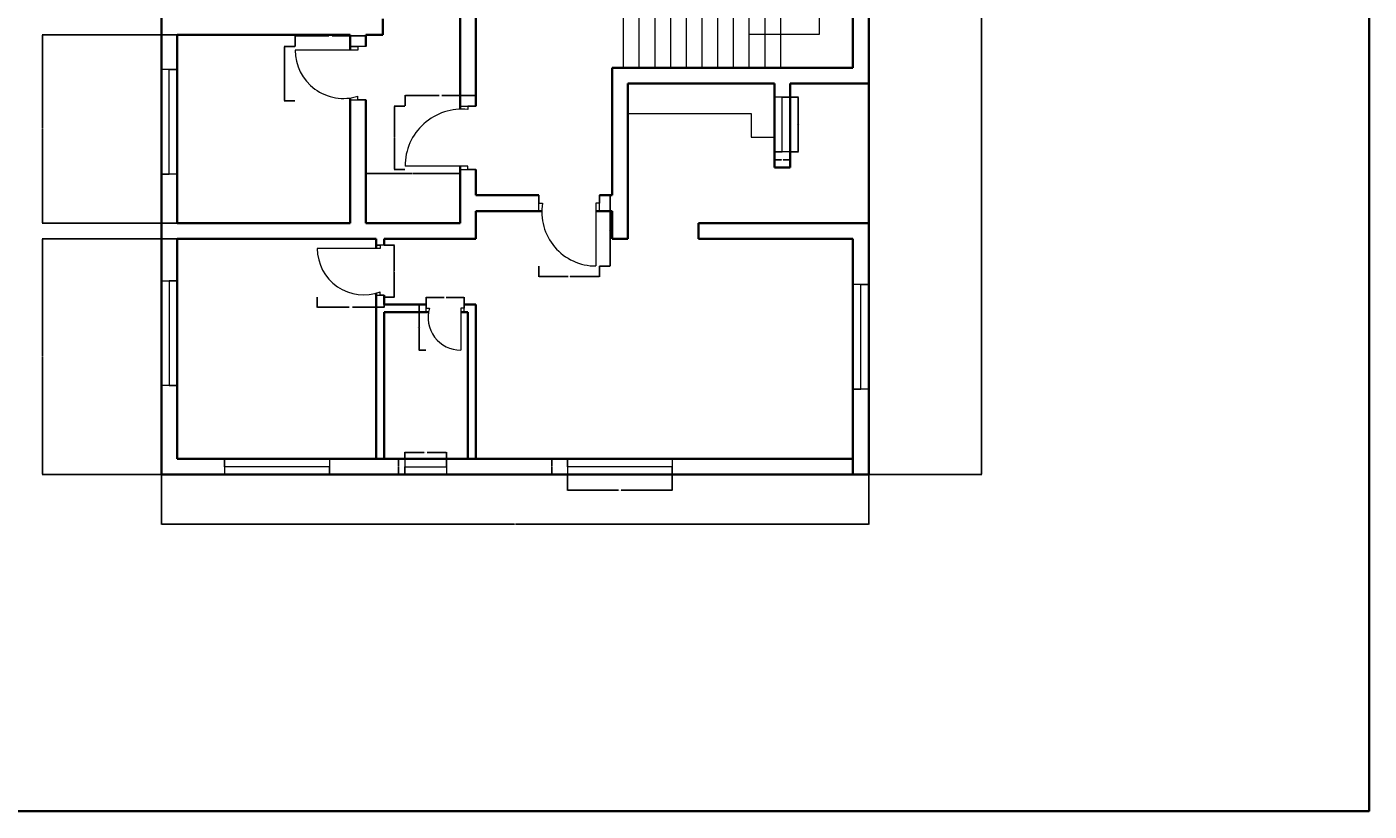
# Model space of a CAD drawing. Units: inches. Extents: x 1955 to 3324, y 980 to 3129.
# Tile 7 of 11: x 2555 to 3324, y 1704 to 2153. Entities that reach past the tile are written whole.
import ezdxf

# ---------------------------------------------------------------- set-up
doc = ezdxf.new("R2010")
doc.units = ezdxf.units.IN
for name, color, linetype, lineweight in [('A-ANNO-DIMS', 2, 'Continuous', 18), ('A-ANNO-TTLB', 7, 'Continuous', 35), ('A-DOOR', 3, 'Continuous', 18), ('A-FLOR-CASE', 8, 'Continuous', 18), ('A-FLOR-STRS', 7, 'Continuous', 18), ('A-GLAZ', 4, 'Continuous', 18), ('A-WALL', 7, 'Continuous', 35)]:
    doc.layers.add(name, color=color, linetype=linetype, lineweight=lineweight)
doc.styles.get("Standard").update_dxf_attribs({"font": 'arial.ttf'})
doc.dimstyles.get("Standard").update_dxf_attribs({"dimtxt": 0.18, "dimasz": 0.18, "dimexe": 0.18, "dimexo": 0.0625, "dimgap": 0.09, "dimtad": 0, "dimtih": 1, "dimtoh": 1, "dimdec": 4, "dimzin": 0, "dimdsep": 46, "dimtxsty": 'Standard', "dimcen": 0.09, "dimadec": 0, "dimazin": 0, "dimtfac": 1, "dimtdec": 4, "dimtofl": 0, "dimtmove": 0, "dimatfit": 3, "dimfxl": 1, "dimtolj": 1, "dimtzin": 0, "dimarcsym": 0})

# ---------------------------------------------------------------- blocks, each defined once
blk = doc.blocks.new('DOOR-UNIT-W')
for p, q in [((31.5, 36.35), (40.5, 36.35)), ((40.5, 36.35), (36, 36.35)), ((36, 36.35), (36, 34.35)), ((36, 2), (0, 2)), ((31.5, 0), (40.5, 0)), ((36, 0), (36, 2)), ((40.5, 0), (36, 0))]:
    blk.add_line(p, q)
blk.add_arc((32.53, 2), 32.53, 83.87992, 180)
blk = doc.blocks.new('DOOR-BED-S')
for p, q in [((36, 26.66), (0, 26.66)), ((38.25, 28.66), (33.75, 28.66)), ((33.75, 28.66), (36, 28.66)), ((36, 28.66), (36, 26.66)), ((36, 0), (36, 2)), ((33.75, 0), (38.25, 0)), ((38.25, 0), (36, 0))]:
    blk.add_line(p, q)
blk.add_arc((26.45, 26.66), 26.45, 180, 291.17181)
blk = doc.blocks.new('DOOR-WC-S')
for p, q in [((0, 21.75), (0, 26.25)), ((0, 26.25), (0, 24)), ((0, 24), (2, 24)), ((21.9, 24), (19.9, 24)), ((19.9, 24), (19.9, 0)), ((21.9, 21.75), (21.9, 26.25)), ((21.9, 26.25), (21.9, 24))]:
    blk.add_line(p, q)
blk.add_arc((19.9, 18.68), 18.68, 163.43907, 270)
blk = doc.blocks.new('DOOR-UNIT-S')
for p, q in [((0, 31.5), (0, 40.5)), ((0, 40.5), (0, 36)), ((34.6, 31.5), (34.6, 40.5)), ((34.6, 40.5), (34.6, 36)), ((0, 36), (2, 36)), ((34.6, 36), (32.6, 36)), ((32.6, 36), (32.6, 0))]:
    blk.add_line(p, q)
blk.add_arc((32.6, 31.01), 31.01, 170.73008, 270)
blk = doc.blocks.new('DOOR-BED-W')
for p, q in [((36, 28.47), (0, 28.47)), ((40.5, 30.47), (31.5, 30.47)), ((31.5, 30.47), (36, 30.47)), ((36, 30.47), (36, 28.47)), ((31.5, 0), (40.5, 0)), ((36, 0), (36, 2)), ((40.5, 0), (36, 0))]:
    blk.add_line(p, q)
blk.add_arc((27.73, 28.47), 27.73, 180, 287.3494)
blk = doc.blocks.new('WIN-PLAN-60-A')
for p, q in [((0, 60), (9, 60)), ((9, 60), (4.5, 60)), ((4.5, 60), (4.5, 0)), ((4.5, 0), (0, 0)), ((0, 0), (9, 0))]:
    blk.add_line(p, q)
blk = doc.blocks.new('WIN-PLAN-60-B')
for p, q in [((0, 0), (0, 9)), ((0, 9), (0, 4.5)), ((60, 4.5), (60, 9)), ((60, 9), (60, 0)), ((0, 4.5), (60, 4.5))]:
    blk.add_line(p, q)
blk = doc.blocks.new('WIN-PLAN-24-A')
for p, q in [((0, 9), (0, 0)), ((24, 4.5), (24, 9)), ((24, 9), (24, 0)), ((0, 0), (0, 4.5)), ((0, 4.5), (24, 4.5))]:
    blk.add_line(p, q)
blk = doc.blocks.new('WIN-PLAN-31')
for p, q in [((0, 31.31), (9, 31.31)), ((9, 31.31), (4.5, 31.31)), ((4.5, 31.31), (4.5, 0)), ((4.5, 0), (0, 0)), ((0, 0), (9, 0))]:
    blk.add_line(p, q)
blk = doc.blocks.new('COUNTER-L-S')
for p, q in [((0, 13.55), (70.65, 13.55)), ((70.65, 13.55), (70.65, 0)), ((70.65, 0), (83.99, 0))]:
    blk.add_line(p, q)
blk = doc.blocks.new('STAIR-RETURN-FLIGHT')
for p, q in [((17.37, 47), (17.37, 94)), ((17.37, 94), (17.37, 0)), ((26.37, 94), (26.37, 0)), ((35.37, 94), (35.37, 0)), ((44.37, 94), (44.37, 0)), ((53.37, 94), (53.37, 0)), ((62.37, 94), (62.37, 0)), ((71.37, 94), (71.37, 0)), ((80.37, 94), (80.37, 0)), ((89.37, 94), (89.37, 0)), ((98.37, 94), (98.37, 0)), ((107.37, 94), (107.37, 0)), ((0, 68.91), (129.63, 68.91)), ((129.63, 68.91), (129.63, 19.03)), ((107.37, 47), (17.37, 47)), ((129.63, 19.03), (89.37, 19.03))]:
    blk.add_line(p, q)
blk = doc.blocks.new('*D31')
at = {"layer": 'A-ANNO-DIMS', "color": 0, "lineweight": -2, "transparency": 16777216}
for p, q in [((2864.86, 1896.44), (2864.86, 1887.32)), ((2924.86, 1896.44), (2924.86, 1887.32)), ((2865.04, 1887.5), (2894.01, 1887.5)), ((2924.68, 1887.5), (2895.7, 1887.5))]:
    blk.add_line(p, q, dxfattribs=at)
at = {"layer": 'A-ANNO-DIMS', "color": 0, "transparency": 16777216}
for points in [[(2865.04, 1887.53), (2865.04, 1887.47), (2864.86, 1887.5)], [(2924.68, 1887.53), (2924.68, 1887.47), (2924.86, 1887.5)]]:
    blk.add_solid(points, dxfattribs=at)
at = {"layer": 'Defpoints', "color": 0, "transparency": 16777216}
for p in [(2864.86, 1896.5), (2924.86, 1896.5), (2924.86, 1887.5)]:
    blk.add_point(p, dxfattribs=at)
at = {"layer": 'A-ANNO-DIMS', "color": 0, "transparency": 16777216, "insert": (2894.86, 1887.5), "char_height": 0.18, "attachment_point": 5}
blk.add_mtext('\\A1;WIN. 60 TYP.', dxfattribs=at)
blk = doc.blocks.new('*D32')
at = {"layer": 'A-ANNO-DIMS', "color": 0, "lineweight": -2, "transparency": 16777216}
for p, q in [((2864.79, 1905.5), (2855.68, 1905.5)), ((2855.86, 1905.32), (2855.86, 1901.19)), ((2855.86, 1896.68), (2855.86, 1900.82)), ((2864.79, 1896.5), (2855.68, 1896.5))]:
    blk.add_line(p, q, dxfattribs=at)
at = {"layer": 'A-ANNO-DIMS', "color": 0, "transparency": 16777216}
for points in [[(2855.83, 1905.32), (2855.89, 1905.32), (2855.86, 1905.5)], [(2855.83, 1896.68), (2855.89, 1896.68), (2855.86, 1896.5)]]:
    blk.add_solid(points, dxfattribs=at)
at = {"layer": 'Defpoints', "color": 0, "transparency": 16777216}
for p in [(2864.86, 1905.5), (2855.86, 1896.5), (2864.86, 1896.5)]:
    blk.add_point(p, dxfattribs=at)
at = {"layer": 'A-ANNO-DIMS', "color": 0, "transparency": 16777216, "insert": (2855.86, 1901), "char_height": 0.18, "attachment_point": 5}
blk.add_mtext('\\A1;9 TYP.', dxfattribs=at)
blk = doc.blocks.new('*D37')
at = {"layer": 'A-ANNO-DIMS', "color": 0, "lineweight": -2, "transparency": 16777216}
for p, q in [((2771.65, 1905.57), (2771.65, 1909.28)), ((2771.83, 1909.1), (2782.8, 1909.1)), ((2795.47, 1909.1), (2784.49, 1909.1)), ((2795.65, 1905.57), (2795.65, 1909.28))]:
    blk.add_line(p, q, dxfattribs=at)
at = {"layer": 'A-ANNO-DIMS', "color": 0, "transparency": 16777216}
for points in [[(2771.83, 1909.13), (2771.83, 1909.07), (2771.65, 1909.1)], [(2795.47, 1909.13), (2795.47, 1909.07), (2795.65, 1909.1)]]:
    blk.add_solid(points, dxfattribs=at)
at = {"layer": 'Defpoints', "color": 0, "transparency": 16777216}
for p in [(2795.65, 1909.1), (2771.65, 1905.5), (2795.65, 1905.5)]:
    blk.add_point(p, dxfattribs=at)
at = {"layer": 'A-ANNO-DIMS', "color": 0, "transparency": 16777216, "insert": (2783.65, 1909.1), "char_height": 0.18, "attachment_point": 5}
blk.add_mtext('\\A1;WIN. 24 TYP.', dxfattribs=at)
blk = doc.blocks.new('*D38')
at = {"layer": 'A-ANNO-DIMS', "color": 0, "lineweight": -2, "transparency": 16777216}
for p, q in [((2771.59, 1905.5), (2767.87, 1905.5)), ((2768.05, 1905.32), (2768.05, 1901.19)), ((2768.05, 1896.68), (2768.05, 1900.82)), ((2771.59, 1896.5), (2767.87, 1896.5))]:
    blk.add_line(p, q, dxfattribs=at)
at = {"layer": 'A-ANNO-DIMS', "color": 0, "transparency": 16777216}
for points in [[(2768.02, 1905.32), (2768.08, 1905.32), (2768.05, 1905.5)], [(2768.02, 1896.68), (2768.08, 1896.68), (2768.05, 1896.5)]]:
    blk.add_solid(points, dxfattribs=at)
at = {"layer": 'Defpoints', "color": 0, "transparency": 16777216}
for p in [(2768.05, 1905.5), (2771.65, 1905.5), (2771.65, 1896.5)]:
    blk.add_point(p, dxfattribs=at)
at = {"layer": 'A-ANNO-DIMS', "color": 0, "transparency": 16777216, "insert": (2768.05, 1901), "char_height": 0.18, "attachment_point": 5}
blk.add_mtext('\\A1;9 TYP.', dxfattribs=at)
blk = doc.blocks.new('*D45')
at = {"layer": 'A-ANNO-DIMS', "color": 0, "lineweight": -2, "transparency": 16777216}
for p, q in [((2992.43, 2112.79), (2997.25, 2112.79)), ((2997.07, 2112.61), (2997.07, 2097.32)), ((2997.07, 2081.67), (2997.07, 2096.96)), ((2992.43, 2081.49), (2997.25, 2081.49))]:
    blk.add_line(p, q, dxfattribs=at)
at = {"layer": 'A-ANNO-DIMS', "color": 0, "transparency": 16777216}
for points in [[(2997.04, 2112.61), (2997.1, 2112.61), (2997.07, 2112.79)], [(2997.04, 2081.67), (2997.1, 2081.67), (2997.07, 2081.49)]]:
    blk.add_solid(points, dxfattribs=at)
at = {"layer": 'Defpoints', "color": 0, "transparency": 16777216}
for p in [(2992.37, 2112.79), (2992.37, 2081.49), (2997.07, 2081.49)]:
    blk.add_point(p, dxfattribs=at)
at = {"layer": 'A-ANNO-DIMS', "color": 0, "transparency": 16777216, "insert": (2997.07, 2097.14), "char_height": 0.18, "attachment_point": 5}
blk.add_mtext('\\A1;WIN. 31 TYP.', dxfattribs=at)
blk = doc.blocks.new('*D46')
at = {"layer": 'A-ANNO-DIMS', "color": 0, "lineweight": -2, "transparency": 16777216}
for p, q in [((2983.37, 2081.42), (2983.37, 2076.61)), ((2983.55, 2076.79), (2987.41, 2076.79)), ((2992.19, 2076.79), (2988.33, 2076.79)), ((2992.37, 2081.42), (2992.37, 2076.61))]:
    blk.add_line(p, q, dxfattribs=at)
at = {"layer": 'A-ANNO-DIMS', "color": 0, "transparency": 16777216}
for points in [[(2983.55, 2076.82), (2983.55, 2076.76), (2983.37, 2076.79)], [(2992.19, 2076.82), (2992.19, 2076.76), (2992.37, 2076.79)]]:
    blk.add_solid(points, dxfattribs=at)
at = {"layer": 'Defpoints', "color": 0, "transparency": 16777216}
for p in [(2983.37, 2081.49), (2983.37, 2076.79), (2992.37, 2081.49)]:
    blk.add_point(p, dxfattribs=at)
at = {"layer": 'A-ANNO-DIMS', "color": 0, "transparency": 16777216, "insert": (2987.87, 2076.79), "char_height": 0.18, "attachment_point": 5}
blk.add_mtext('\\A1;9 TYP.', dxfattribs=at)
blk = doc.blocks.new('*D63')
at = {"layer": 'A-ANNO-DIMS', "color": 0, "lineweight": -2, "transparency": 16777216}
for p, q in [((2771.87, 2107.68), (2771.87, 2113.87)), ((2772.05, 2113.69), (2791.34, 2113.69)), ((2812.19, 2113.69), (2792.89, 2113.69)), ((2812.37, 2107.68), (2812.37, 2113.87))]:
    blk.add_line(p, q, dxfattribs=at)
at = {"layer": 'A-ANNO-DIMS', "color": 0, "transparency": 16777216}
for points in [[(2772.05, 2113.72), (2772.05, 2113.66), (2771.87, 2113.69)], [(2812.19, 2113.72), (2812.19, 2113.66), (2812.37, 2113.69)]]:
    blk.add_solid(points, dxfattribs=at)
at = {"layer": 'Defpoints', "color": 0, "transparency": 16777216}
for p in [(2771.87, 2107.62), (2812.37, 2113.69), (2812.37, 2107.62)]:
    blk.add_point(p, dxfattribs=at)
at = {"layer": 'A-ANNO-DIMS', "color": 0, "transparency": 16777216, "insert": (2792.12, 2113.69), "char_height": 0.18, "attachment_point": 5}
blk.add_mtext('\\A1;DR. 41 TYP.', dxfattribs=at)
blk = doc.blocks.new('*D64')
at = {"layer": 'A-ANNO-DIMS', "color": 0, "lineweight": -2, "transparency": 16777216}
for p, q in [((2771.81, 2107.62), (2765.61, 2107.62)), ((2765.79, 2107.44), (2765.79, 2089.63)), ((2765.79, 2071.45), (2765.79, 2089.26)), ((2771.81, 2071.27), (2765.61, 2071.27))]:
    blk.add_line(p, q, dxfattribs=at)
at = {"layer": 'A-ANNO-DIMS', "color": 0, "transparency": 16777216}
for points in [[(2765.76, 2107.44), (2765.82, 2107.44), (2765.79, 2107.62)], [(2765.76, 2071.45), (2765.82, 2071.45), (2765.79, 2071.27)]]:
    blk.add_solid(points, dxfattribs=at)
at = {"layer": 'Defpoints', "color": 0, "transparency": 16777216}
for p in [(2765.79, 2107.62), (2771.87, 2107.62), (2771.87, 2071.27)]:
    blk.add_point(p, dxfattribs=at)
at = {"layer": 'A-ANNO-DIMS', "color": 0, "transparency": 16777216, "insert": (2765.79, 2089.45), "char_height": 0.18, "attachment_point": 5}
blk.add_mtext('\\A1;36 TYP.', dxfattribs=at)
blk = doc.blocks.new('*D65')
at = {"layer": 'A-ANNO-DIMS', "color": 0, "lineweight": -2, "transparency": 16777216}
for p, q in [((2721.62, 1998.05), (2721.62, 1992.2)), ((2721.8, 1992.38), (2739.81, 1992.38)), ((2759.69, 1992.38), (2741.68, 1992.38)), ((2759.87, 1998.05), (2759.87, 1992.2))]:
    blk.add_line(p, q, dxfattribs=at)
at = {"layer": 'A-ANNO-DIMS', "color": 0, "transparency": 16777216}
for points in [[(2721.8, 1992.41), (2721.8, 1992.35), (2721.62, 1992.38)], [(2759.69, 1992.41), (2759.69, 1992.35), (2759.87, 1992.38)]]:
    blk.add_solid(points, dxfattribs=at)
at = {"layer": 'Defpoints', "color": 0, "transparency": 16777216}
for p in [(2721.62, 1998.11), (2759.87, 1998.11), (2759.87, 1992.38)]:
    blk.add_point(p, dxfattribs=at)
at = {"layer": 'A-ANNO-DIMS', "color": 0, "transparency": 16777216, "insert": (2740.74, 1992.38), "char_height": 0.18, "attachment_point": 5}
blk.add_mtext('\\A1;DOOR 38 TYP.', dxfattribs=at)
blk = doc.blocks.new('*D66')
at = {"layer": 'A-ANNO-DIMS', "color": 0, "lineweight": -2, "transparency": 16777216}
for p, q in [((2759.93, 2027.93), (2765.79, 2027.93)), ((2765.61, 2027.75), (2765.61, 2013.2)), ((2765.61, 1998.29), (2765.61, 2012.84)), ((2759.93, 1998.11), (2765.79, 1998.11))]:
    blk.add_line(p, q, dxfattribs=at)
at = {"layer": 'A-ANNO-DIMS', "color": 0, "transparency": 16777216}
for points in [[(2765.58, 2027.75), (2765.64, 2027.75), (2765.61, 2027.93)], [(2765.58, 1998.29), (2765.64, 1998.29), (2765.61, 1998.11)]]:
    blk.add_solid(points, dxfattribs=at)
at = {"layer": 'Defpoints', "color": 0, "transparency": 16777216}
for p in [(2759.87, 2027.93), (2765.61, 2027.93), (2759.87, 1998.11)]:
    blk.add_point(p, dxfattribs=at)
at = {"layer": 'A-ANNO-DIMS', "color": 0, "transparency": 16777216, "insert": (2765.61, 2013.02), "char_height": 0.18, "attachment_point": 5}
blk.add_mtext('\\A1;30 TYP.', dxfattribs=at)
blk = doc.blocks.new('*D67')
at = {"layer": 'A-ANNO-DIMS', "color": 0, "lineweight": -2, "transparency": 16777216}
for p, q in [((2783.81, 1994), (2779.75, 1994)), ((2779.93, 1993.82), (2779.93, 1981.06)), ((2779.93, 1967.93), (2779.93, 1980.7)), ((2783.81, 1967.75), (2779.75, 1967.75))]:
    blk.add_line(p, q, dxfattribs=at)
at = {"layer": 'A-ANNO-DIMS', "color": 0, "transparency": 16777216}
for points in [[(2779.9, 1993.82), (2779.96, 1993.82), (2779.93, 1994)], [(2779.9, 1967.93), (2779.96, 1967.93), (2779.93, 1967.75)]]:
    blk.add_solid(points, dxfattribs=at)
at = {"layer": 'Defpoints', "color": 0, "transparency": 16777216}
for p in [(2779.93, 1994), (2783.87, 1994), (2783.87, 1967.75)]:
    blk.add_point(p, dxfattribs=at)
at = {"layer": 'A-ANNO-DIMS', "color": 0, "transparency": 16777216, "insert": (2779.93, 1980.88), "char_height": 0.18, "attachment_point": 5}
blk.add_mtext('\\A1;DOOR 26 TYP.', dxfattribs=at)
blk = doc.blocks.new('*D68')
at = {"layer": 'A-ANNO-DIMS', "color": 0, "lineweight": -2, "transparency": 16777216}
for p, q in [((2783.87, 1994.07), (2783.87, 1998.12)), ((2784.05, 1997.94), (2794.29, 1997.94)), ((2805.59, 1997.94), (2795.35, 1997.94)), ((2805.77, 1994.07), (2805.77, 1998.12))]:
    blk.add_line(p, q, dxfattribs=at)
at = {"layer": 'A-ANNO-DIMS', "color": 0, "transparency": 16777216}
for points in [[(2784.05, 1997.97), (2784.05, 1997.91), (2783.87, 1997.94)], [(2805.59, 1997.97), (2805.59, 1997.91), (2805.77, 1997.94)]]:
    blk.add_solid(points, dxfattribs=at)
at = {"layer": 'Defpoints', "color": 0, "transparency": 16777216}
for p in [(2783.87, 1994), (2805.77, 1997.94), (2805.77, 1994)]:
    blk.add_point(p, dxfattribs=at)
at = {"layer": 'A-ANNO-DIMS', "color": 0, "transparency": 16777216, "insert": (2794.82, 1997.94), "char_height": 0.18, "attachment_point": 5}
blk.add_mtext('\\A1;22 TYP.', dxfattribs=at)
blk = doc.blocks.new('*D73')
at = {"layer": 'A-ANNO-DIMS', "color": 0, "lineweight": -2, "transparency": 16777216}
for p, q in [((2883.23, 2056.49), (2889.42, 2056.49)), ((2889.24, 2056.31), (2889.24, 2036.42)), ((2889.24, 2016.17), (2889.24, 2036.06)), ((2883.23, 2015.99), (2889.42, 2015.99))]:
    blk.add_line(p, q, dxfattribs=at)
at = {"layer": 'A-ANNO-DIMS', "color": 0, "transparency": 16777216}
for points in [[(2889.21, 2056.31), (2889.27, 2056.31), (2889.24, 2056.49)], [(2889.21, 2016.17), (2889.27, 2016.17), (2889.24, 2015.99)]]:
    blk.add_solid(points, dxfattribs=at)
at = {"layer": 'Defpoints', "color": 0, "transparency": 16777216}
for p in [(2883.17, 2056.49), (2889.24, 2056.49), (2883.17, 2015.99)]:
    blk.add_point(p, dxfattribs=at)
at = {"layer": 'A-ANNO-DIMS', "color": 0, "transparency": 16777216, "insert": (2889.24, 2036.24), "char_height": 0.18, "attachment_point": 5}
blk.add_mtext('\\A1;ENTRY 41 TYP.', dxfattribs=at)
blk = doc.blocks.new('*D74')
at = {"layer": 'A-ANNO-DIMS', "color": 0, "lineweight": -2, "transparency": 16777216}
for p, q in [((2848.57, 2015.93), (2848.57, 2009.74)), ((2883.17, 2015.93), (2883.17, 2009.74)), ((2848.75, 2009.92), (2865.34, 2009.92)), ((2882.99, 2009.92), (2866.4, 2009.92))]:
    blk.add_line(p, q, dxfattribs=at)
at = {"layer": 'A-ANNO-DIMS', "color": 0, "transparency": 16777216}
for points in [[(2848.75, 2009.95), (2848.75, 2009.89), (2848.57, 2009.92)], [(2882.99, 2009.95), (2882.99, 2009.89), (2883.17, 2009.92)]]:
    blk.add_solid(points, dxfattribs=at)
at = {"layer": 'Defpoints', "color": 0, "transparency": 16777216}
for p in [(2848.57, 2015.99), (2883.17, 2015.99), (2883.17, 2009.92)]:
    blk.add_point(p, dxfattribs=at)
at = {"layer": 'A-ANNO-DIMS', "color": 0, "transparency": 16777216, "insert": (2865.87, 2009.92), "char_height": 0.18, "attachment_point": 5}
blk.add_mtext('\\A1;35 TYP.', dxfattribs=at)
blk = doc.blocks.new('*D75')
at = {"layer": 'A-ANNO-DIMS', "color": 0, "lineweight": -2, "transparency": 16777216}
for p, q in [((2708.87, 2141.79), (2708.87, 2147.98)), ((2709.05, 2147.8), (2728.18, 2147.8)), ((2749.19, 2147.8), (2730.06, 2147.8)), ((2749.37, 2141.79), (2749.37, 2147.98))]:
    blk.add_line(p, q, dxfattribs=at)
at = {"layer": 'A-ANNO-DIMS', "color": 0, "transparency": 16777216}
for points in [[(2709.05, 2147.83), (2709.05, 2147.77), (2708.87, 2147.8)], [(2749.19, 2147.83), (2749.19, 2147.77), (2749.37, 2147.8)]]:
    blk.add_solid(points, dxfattribs=at)
at = {"layer": 'Defpoints', "color": 0, "transparency": 16777216}
for p in [(2749.37, 2147.8), (2708.87, 2141.73), (2749.37, 2141.73)]:
    blk.add_point(p, dxfattribs=at)
at = {"layer": 'A-ANNO-DIMS', "color": 0, "transparency": 16777216, "insert": (2729.12, 2147.8), "char_height": 0.18, "attachment_point": 5}
blk.add_mtext('\\A1;DOOR 41 TYP.', dxfattribs=at)
blk = doc.blocks.new('*D76')
at = {"layer": 'A-ANNO-DIMS', "color": 0, "lineweight": -2, "transparency": 16777216}
for p, q in [((2708.81, 2141.73), (2702.61, 2141.73)), ((2702.79, 2141.55), (2702.79, 2126.36)), ((2702.79, 2110.81), (2702.79, 2125.99)), ((2708.81, 2110.63), (2702.61, 2110.63))]:
    blk.add_line(p, q, dxfattribs=at)
at = {"layer": 'A-ANNO-DIMS', "color": 0, "transparency": 16777216}
for points in [[(2702.76, 2141.55), (2702.82, 2141.55), (2702.79, 2141.73)], [(2702.76, 2110.81), (2702.82, 2110.81), (2702.79, 2110.63)]]:
    blk.add_solid(points, dxfattribs=at)
at = {"layer": 'Defpoints', "color": 0, "transparency": 16777216}
for p in [(2702.79, 2141.73), (2708.87, 2141.73), (2708.87, 2110.63)]:
    blk.add_point(p, dxfattribs=at)
at = {"layer": 'A-ANNO-DIMS', "color": 0, "transparency": 16777216, "insert": (2702.79, 2126.18), "char_height": 0.18, "attachment_point": 5}
blk.add_mtext('\\A1;31 TYP.', dxfattribs=at)
blk = doc.blocks.new('*D93')
at = {"layer": 'A-ANNO-DIMS', "color": 0, "lineweight": -2, "transparency": 16777216}
for p, q in [((2632.37, 1896.44), (2632.37, 1867.87)), ((3037.37, 1896.44), (3037.37, 1867.87)), ((2632.55, 1868.05), (2834.58, 1868.05)), ((3037.19, 1868.05), (2835.16, 1868.05))]:
    blk.add_line(p, q, dxfattribs=at)
at = {"layer": 'A-ANNO-DIMS', "color": 0, "transparency": 16777216}
for points in [[(2632.55, 1868.08), (2632.55, 1868.02), (2632.37, 1868.05)], [(3037.19, 1868.08), (3037.19, 1868.02), (3037.37, 1868.05)]]:
    blk.add_solid(points, dxfattribs=at)
at = {"layer": 'Defpoints', "color": 0, "transparency": 16777216}
for p in [(2632.37, 1896.5), (3037.37, 1896.5), (3037.37, 1868.05)]:
    blk.add_point(p, dxfattribs=at)
at = {"layer": 'A-ANNO-DIMS', "color": 0, "transparency": 16777216, "insert": (2834.87, 1868.05), "char_height": 0.18, "attachment_point": 5}
blk.add_mtext('\\A1;405', dxfattribs=at)
blk = doc.blocks.new('*D94')
at = {"layer": 'A-ANNO-DIMS', "color": 0, "lineweight": -2, "transparency": 16777216}
for p, q in [((3037.43, 2456.5), (3102.13, 2456.5)), ((3101.95, 2456.32), (3101.95, 2176.69)), ((3101.95, 1896.68), (3101.95, 2176.32)), ((3037.43, 1896.5), (3102.13, 1896.5))]:
    blk.add_line(p, q, dxfattribs=at)
at = {"layer": 'A-ANNO-DIMS', "color": 0, "transparency": 16777216}
for points in [[(3101.92, 2456.32), (3101.98, 2456.32), (3101.95, 2456.5)], [(3101.92, 1896.68), (3101.98, 1896.68), (3101.95, 1896.5)]]:
    blk.add_solid(points, dxfattribs=at)
at = {"layer": 'Defpoints', "color": 0, "transparency": 16777216}
for p in [(3037.37, 2456.5), (3101.95, 2456.5), (3037.37, 1896.5)]:
    blk.add_point(p, dxfattribs=at)
at = {"layer": 'A-ANNO-DIMS', "color": 0, "transparency": 16777216, "insert": (3101.95, 2176.5), "char_height": 0.18, "attachment_point": 5}
blk.add_mtext('\\A1;560', dxfattribs=at)
blk = doc.blocks.new('*D98')
at = {"layer": 'A-ANNO-DIMS', "color": 0, "lineweight": -2, "transparency": 16777216}
for p, q in [((2641.31, 2031.5), (2564.03, 2031.5)), ((2564.21, 2031.32), (2564.21, 1964.19)), ((2564.21, 1896.68), (2564.21, 1963.82)), ((2632.31, 1896.5), (2564.03, 1896.5))]:
    blk.add_line(p, q, dxfattribs=at)
at = {"layer": 'A-ANNO-DIMS', "color": 0, "transparency": 16777216}
for points in [[(2564.18, 2031.32), (2564.24, 2031.32), (2564.21, 2031.5)], [(2564.18, 1896.68), (2564.24, 1896.68), (2564.21, 1896.5)]]:
    blk.add_solid(points, dxfattribs=at)
at = {"layer": 'Defpoints', "color": 0, "transparency": 16777216}
for p in [(2564.21, 2031.5), (2641.37, 2031.5), (2632.37, 1896.5)]:
    blk.add_point(p, dxfattribs=at)
at = {"layer": 'A-ANNO-DIMS', "color": 0, "transparency": 16777216, "insert": (2564.21, 1964), "char_height": 0.18, "attachment_point": 5}
blk.add_mtext('\\A1;135', dxfattribs=at)
blk = doc.blocks.new('*D99')
at = {"layer": 'A-ANNO-DIMS', "color": 0, "lineweight": -2, "transparency": 16777216}
for p, q in [((2641.31, 2148.5), (2564.03, 2148.5)), ((2564.21, 2148.32), (2564.21, 2094.69)), ((2564.21, 2040.68), (2564.21, 2094.32)), ((2641.31, 2040.5), (2564.03, 2040.5))]:
    blk.add_line(p, q, dxfattribs=at)
at = {"layer": 'A-ANNO-DIMS', "color": 0, "transparency": 16777216}
for points in [[(2564.18, 2148.32), (2564.24, 2148.32), (2564.21, 2148.5)], [(2564.18, 2040.68), (2564.24, 2040.68), (2564.21, 2040.5)]]:
    blk.add_solid(points, dxfattribs=at)
at = {"layer": 'Defpoints', "color": 0, "transparency": 16777216}
for p in [(2564.21, 2148.5), (2641.37, 2148.5), (2641.37, 2040.5)]:
    blk.add_point(p, dxfattribs=at)
at = {"layer": 'A-ANNO-DIMS', "color": 0, "transparency": 16777216, "insert": (2564.21, 2094.5), "char_height": 0.18, "attachment_point": 5}
blk.add_mtext('\\A1;108', dxfattribs=at)
blk = doc.blocks.new('*D101')
at = {"layer": 'A-ANNO-DIMS', "color": 0, "lineweight": -2, "transparency": 16777216}
for p, q in [((2749.37, 2040.57), (2749.37, 2069.13)), ((2749.55, 2068.95), (2776.15, 2068.95)), ((2803.19, 2068.95), (2776.59, 2068.95)), ((2803.37, 2040.57), (2803.37, 2069.13))]:
    blk.add_line(p, q, dxfattribs=at)
at = {"layer": 'A-ANNO-DIMS', "color": 0, "transparency": 16777216}
for points in [[(2749.55, 2068.98), (2749.55, 2068.92), (2749.37, 2068.95)], [(2803.19, 2068.98), (2803.19, 2068.92), (2803.37, 2068.95)]]:
    blk.add_solid(points, dxfattribs=at)
at = {"layer": 'Defpoints', "color": 0, "transparency": 16777216}
for p in [(2803.37, 2068.95), (2749.37, 2040.5), (2803.37, 2040.5)]:
    blk.add_point(p, dxfattribs=at)
at = {"layer": 'A-ANNO-DIMS', "color": 0, "transparency": 16777216, "insert": (2776.37, 2068.95), "char_height": 0.18, "attachment_point": 5}
blk.add_mtext('\\A1;54', dxfattribs=at)

msp = doc.modelspace()

# ---------------------------------------------------------------- linework, layer by layer
at = {"layer": 'A-ANNO-TTLB'}
msp.add_lwpolyline([(1954.5391, 3128.9103), (3323.9705, 3128.9103), (3323.9705, 1703.6826), (1954.5391, 1703.6826)], close=True, dxfattribs=at)
at = {"layer": 'A-WALL'}
for p, q in [((2632.3694, 1896.5037), (2632.3694, 2456.5037)), ((3037.3694, 2456.5037), (3037.3694, 1896.5037)), ((2803.3694, 2312.5037), (2803.3694, 2105.7875)), ((2812.3694, 2267.9289), (2812.3694, 2107.6185)), ((3028.3694, 2223.5037), (3028.3694, 2129.5037)), ((2759.0757, 2157.5037), (2759.0757, 2148.5037)), ((2740.3694, 2148.5037), (2641.3694, 2148.5037)), ((2641.3694, 2040.5037), (2641.3694, 2148.5037)), ((2641.3694, 2148.5037), (2740.3694, 2148.5037)), ((2740.3694, 2139.7262), (2740.3694, 2148.5037)), ((2759.0757, 2148.5037), (2749.3694, 2148.5037)), ((2749.3694, 2148.5037), (2749.3694, 2141.7262)), ((2890.381, 2129.5037), (2890.381, 2056.4936)), ((2909.3694, 2129.5037), (2890.381, 2129.5037)), ((2983.3694, 2129.5037), (2909.3694, 2129.5037)), ((3028.3694, 2129.5037), (2983.3694, 2129.5037)), ((3037.3694, 2120.5037), (3037.3694, 2129.5037)), ((2899.381, 2031.5037), (2899.381, 2120.5037)), ((2983.3694, 2120.5037), (2899.381, 2120.5037)), ((2983.3694, 2120.5037), (2983.3694, 2082.2622)), ((2992.3694, 2082.2622), (2992.3694, 2120.5037)), ((2992.3694, 2120.5037), (3037.3694, 2120.5037)), ((2740.3694, 2040.5037), (2740.3694, 2112.2528)), ((2749.3694, 2111.2571), (2749.3694, 2040.5037)), ((2983.3694, 2082.2622), (2983.3694, 2072.5144)), ((2992.3694, 2072.5144), (2992.3694, 2082.2622)), ((2803.3694, 2073.2722), (2803.3694, 2040.5037)), ((2812.3694, 2071.2722), (2812.3694, 2056.4936)), ((2983.3694, 2072.5144), (2992.3694, 2072.5144)), ((2812.3694, 2056.4936), (2848.5681, 2056.4936)), ((2883.1687, 2056.4936), (2890.381, 2056.4936)), ((2812.3694, 2047.4936), (2812.3694, 2031.5037)), ((2850.1672, 2047.4936), (2812.3694, 2047.4936)), ((2890.381, 2047.4936), (2881.1687, 2047.4936)), ((2890.381, 2047.4936), (2890.381, 2031.5037)), ((2740.3694, 2040.5037), (2641.3694, 2040.5037)), ((2803.3694, 2040.5037), (2749.3694, 2040.5037)), ((2939.9856, 2031.5037), (2939.9856, 2040.5037)), ((2939.9856, 2040.5037), (3028.3694, 2040.5037)), ((3037.3694, 2040.5037), (2992.3694, 2040.5037)), ((2755.3694, 2031.5037), (2641.3694, 2031.5037)), ((2641.3694, 1905.5037), (2641.3694, 2031.5037)), ((2755.3694, 2025.9287), (2755.3694, 2031.5037)), ((2803.3694, 2031.5037), (2759.8694, 2031.5037)), ((2759.8694, 2031.5037), (2759.8694, 2027.9287)), ((2803.3694, 2031.5037), (2812.3694, 2031.5037)), ((2812.3694, 2031.5037), (2807.8694, 2031.5037)), ((2899.381, 2031.5037), (2890.381, 2031.5037)), ((3028.3694, 2031.5037), (2939.9856, 2031.5037)), ((3028.3694, 2031.5037), (3028.3694, 1896.5037)), ((3028.3694, 1905.5037), (3028.3694, 2031.5037)), ((2755.3694, 1994.0037), (2755.3694, 2000.5088)), ((2759.8694, 1999.266), (2759.8694, 1994.0037)), ((2755.3694, 1994.0037), (2755.3694, 1905.5037)), ((2783.8694, 1994.0037), (2759.8694, 1994.0037)), ((2812.3694, 1994.0037), (2805.7711, 1994.0037)), ((2812.3694, 1994.0037), (2812.3694, 1905.5037)), ((2812.3694, 1989.5037), (2812.3694, 1994.0037)), ((2759.8694, 1905.5037), (2759.8694, 1989.5037)), ((2759.8694, 1989.5037), (2785.3492, 1989.5037)), ((2803.7711, 1989.5037), (2807.8694, 1989.5037)), ((2807.8694, 1989.5037), (2807.8694, 1905.5037)), ((3028.3694, 1905.5037), (2641.3694, 1905.5037)), ((2807.8694, 1905.5037), (2759.8694, 1905.5037)), ((2890.381, 1905.5037), (2899.381, 1905.5037)), ((3037.3694, 1896.5037), (2632.3694, 1896.5037)), ((2632.3694, 1896.5037), (2641.3694, 1896.5037))]:
    msp.add_line(p, q, dxfattribs=at)

# ---------------------------------------------------------------- block references
at = {"layer": 'A-DOOR'}
for name, p in [('DOOR-BED-W', (2708.8691, 2111.257)), ('DOOR-UNIT-W', (2771.8691, 2071.272)), ('DOOR-UNIT-S', (2848.5681, 2015.994)), ('DOOR-BED-S', (2721.6191, 1999.266)), ('DOOR-WC-S', (2783.8691, 1967.754))]:
    msp.add_blockref(name, p, dxfattribs=at)
at = {"layer": 'A-FLOR-CASE'}
msp.add_blockref('COUNTER-L-S', (2899.3811, 2089.764), dxfattribs=at)
at = {"layer": 'A-FLOR-STRS'}
msp.add_blockref('STAIR-RETURN-FLIGHT', (2879.4531, 2129.504), dxfattribs=at)
at = {"layer": 'A-GLAZ'}
for name, p, rotation in [('WIN-PLAN-60-A', (2641.3696, 2128.6375), 180), ('WIN-PLAN-31', (2992.3696, 2112.7919), 180), ('WIN-PLAN-60-B', (2632.3697, 2007.5143), 269.9999999999984), ('WIN-PLAN-60-A', (3037.3696, 2005.3635), 180), ('WIN-PLAN-60-A', (2668.5213, 1905.5039), 270.0000000000003), ('WIN-PLAN-60-A', (2864.8559, 1905.5039), 270.0000000000002)]:
    msp.add_blockref(name, p, dxfattribs=dict(at, rotation=rotation))
msp.add_blockref('WIN-PLAN-24-A', (2771.6481, 1896.504), dxfattribs=at)

# ---------------------------------------------------------------- dimensions: what is measured, and where the dimension line sits
at = {"layer": 'A-ANNO-DIMS'}
for base, p1, p2, picture, middle in [((3101.9479, 2456.5037), (3037.3694, 1896.5037), (3037.3694, 2456.5037), '*D94', (3101.9479, 2176.5037)), ((2564.2095, 2148.5037), (2641.3694, 2040.5037), (2641.3694, 2148.5037), '*D99', (2564.2095, 2094.5037)), ((2564.2095, 2031.5037), (2632.3694, 1896.5037), (2641.3694, 2031.5037), '*D98', (2564.2095, 1964.0037))]:
    dim = msp.add_linear_dim(base=base, p1=p1, p2=p2, angle=90, dimstyle='Standard', override={"dimdec": 0, "dimlfac": 1, "dimrnd": 0, "dimzin": 0, "dimdsep": 46, "dimlunit": 2}, dxfattribs=at)
    dim.commit()
    dim.dimension.update_dxf_attribs({"geometry": picture, "text_midpoint": middle})
for base, p1, p2, text, picture, middle in [((2749.3693614392, 2147.801207789), (2708.8693614392, 2141.726207789), (2749.3693614392, 2141.726207789), 'DOOR <> TYP.', '*D75', (2729.1193614392, 2147.801207789)), ((2812.3693614392, 2113.6934841644), (2771.8693614392, 2107.6184841644), (2812.3693614392, 2107.6184841644), 'DR. <> TYP.', '*D63', (2792.1193614392, 2113.6934841644)), ((2883.1687, 2009.9186), (2848.5681, 2015.9936), (2883.1687, 2015.9936), '<> TYP.', '*D74', (2865.8684, 2009.9186)), ((2759.8694, 1992.3774), (2721.6194, 1998.1149), (2759.8694, 1998.1149), 'DOOR <> TYP.', '*D65', (2740.7444, 1992.3774)), ((2805.7711, 1997.9412), (2783.8694, 1994.0037), (2805.7711, 1994.0037), '<> TYP.', '*D68', (2794.8203, 1997.9412)), ((2795.6483, 1909.1037), (2771.6483, 1905.5037), (2795.6483, 1905.5037), 'WIN. <> TYP.', '*D37', (2783.6483, 1909.1037))]:
    dim = msp.add_linear_dim(base=base, p1=p1, p2=p2, text=text, dimstyle='Standard', override={"dimdec": 0, "dimlfac": 1, "dimrnd": 0, "dimzin": 0, "dimdsep": 46, "dimlunit": 2}, dxfattribs=at)
    dim.commit()
    dim.dimension.update_dxf_attribs({"geometry": picture, "text_midpoint": middle})
for base, p1, p2, angle, text, picture, middle in [((2702.7944, 2141.7262), (2708.8694, 2110.6266), (2708.8694, 2141.7262), 90, '<> TYP.', '*D76', (2702.7944, 2126.1764)), ((2765.7944, 2107.6185), (2771.8694, 2071.2722), (2771.8694, 2107.6185), 90, '<> TYP.', '*D64', (2765.7944, 2089.4453)), ((2997.0652, 2081.4868), (2992.3694, 2112.7921), (2992.3694, 2081.4868), 270, 'WIN. <> TYP.', '*D45', (2997.0652, 2097.1395)), ((2983.3694, 2076.791), (2992.3694, 2081.4868), (2983.3694, 2081.4868), 180, '<> TYP.', '*D46', (2987.8694, 2076.791)), ((2889.2436685528, 2056.4936215608), (2883.1686685528, 2015.9936215608), (2883.1686685528, 2056.4936215608), 90, 'ENTRY <> TYP.', '*D73', (2889.2436685528, 2036.2436215608)), ((2765.6069, 2027.9287), (2759.8694, 1998.1149), (2759.8694, 2027.9287), 90, '<> TYP.', '*D66', (2765.6069, 2013.0218)), ((2779.9319, 1994.0037), (2783.8694, 1967.7537), (2783.8694, 1994.0037), 90, 'DOOR <> TYP.', '*D67', (2779.9319, 1980.8787)), ((2768.0483, 1905.5037), (2771.6483, 1896.5037), (2771.6483, 1905.5037), 90, '<> TYP.', '*D38', (2768.0483, 1901.0037)), ((2855.8555, 1896.5037), (2864.8555, 1905.5037), (2864.8555, 1896.5037), 270, '<> TYP.', '*D32', (2855.8555, 1901.0037)), ((2924.8555, 1887.5037), (2864.8555, 1896.5037), (2924.8555, 1896.5037), 0, 'WIN. <> TYP.', '*D31', (2894.8555, 1887.5037))]:
    dim = msp.add_linear_dim(base=base, p1=p1, p2=p2, angle=angle, text=text, dimstyle='Standard', override={"dimdec": 0, "dimlfac": 1, "dimrnd": 0, "dimzin": 0, "dimdsep": 46, "dimlunit": 2}, dxfattribs=at)
    dim.commit()
    dim.dimension.update_dxf_attribs({"geometry": picture, "text_midpoint": middle})
for base, p1, p2, picture, middle in [((2803.3694, 2068.9537), (2749.3694, 2040.5037), (2803.3694, 2040.5037), '*D101', (2776.3694, 2068.9537)), ((3037.3694, 1868.0537), (2632.3694, 1896.5037), (3037.3694, 1896.5037), '*D93', (2834.8694, 1868.0537))]:
    dim = msp.add_linear_dim(base=base, p1=p1, p2=p2, dimstyle='Standard', override={"dimdec": 0, "dimlfac": 1, "dimrnd": 0, "dimzin": 0, "dimdsep": 46, "dimlunit": 2}, dxfattribs=at)
    dim.commit()
    dim.dimension.update_dxf_attribs({"geometry": picture, "text_midpoint": middle})

doc.saveas('drawing.dxf')
